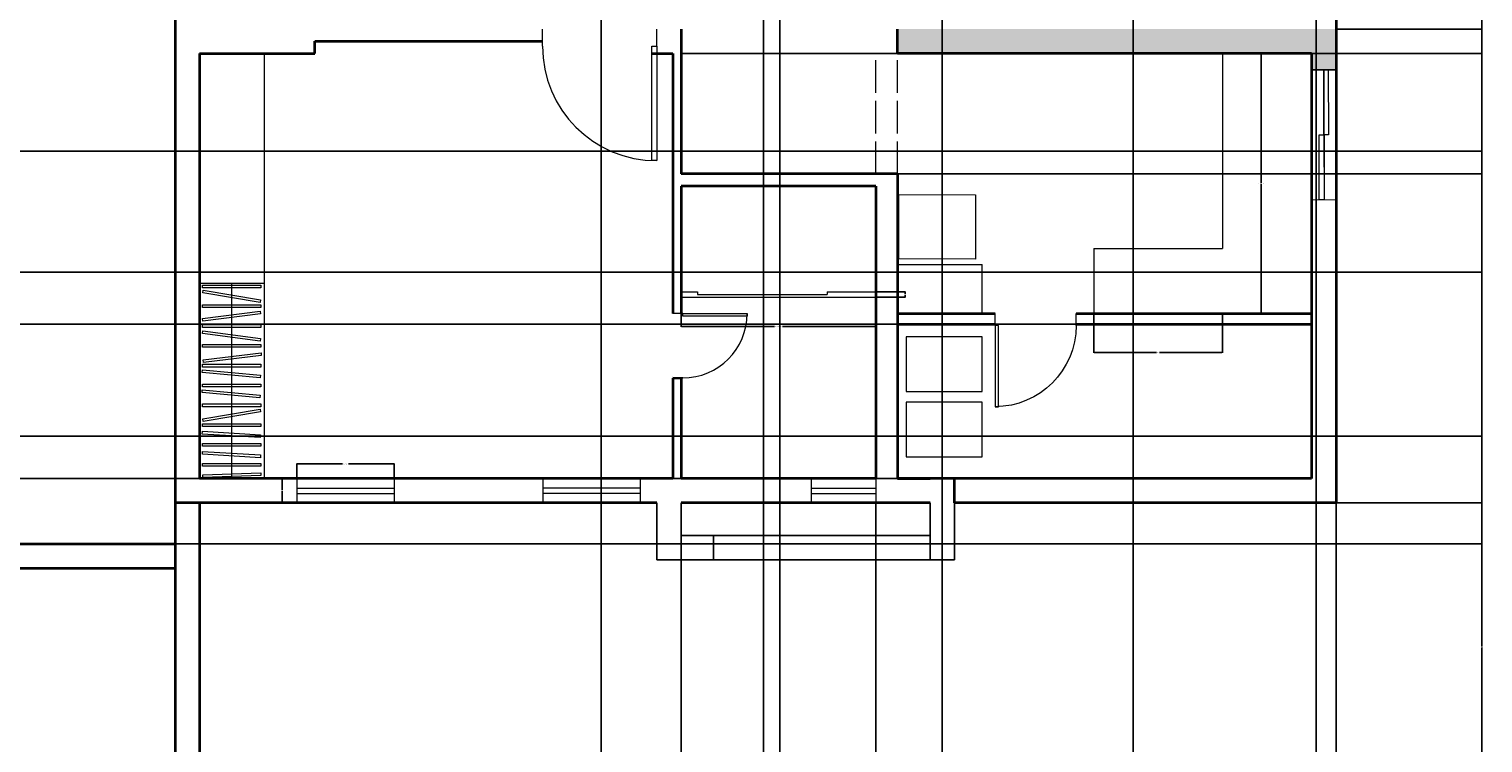
# Model space of a CAD drawing. Units: inches. Extents: x 531915 to 533151, y 849859 to 851471.
# Tile 6 of 7: x 532614 to 533151, y 850858 to 851121. Entities that reach past the tile are written whole.
import ezdxf

# ---------------------------------------------------------------- set-up
doc = ezdxf.new("R2010")
doc.units = ezdxf.units.IN
doc.linetypes.add('ACAD_ISO02W100', pattern=[15, 12, -3])
for name, color, linetype, lineweight in [('A-ANNO-DIMS', 2, 'Continuous', 18), ('A-DOOR', 3, 'Continuous', 18), ('A-FLOR-CASE', 9, 'Continuous', 18), ('A-FLOR-FIXT', 8, 'Continuous', 18), ('A-FLOR-SLAB', 7, 'Continuous', 25), ('A-FURN', 8, 'Continuous', 13), ('A-GLAZ', 4, 'Continuous', 18), ('A-WALL', 7, 'Continuous', 35), ('A-WALL-OVHD', 7, 'ACAD_ISO02W100', 18), ('A-WALL-PATT', 8, 'Continuous', 13)]:
    doc.layers.add(name, color=color, linetype=linetype, lineweight=lineweight)
doc.styles.get("Standard").update_dxf_attribs({"font": 'arial.ttf'})
doc.dimstyles.get("Standard").update_dxf_attribs({"dimtxt": 0.18, "dimasz": 0.18, "dimexe": 0.18, "dimexo": 0.0625, "dimgap": 0.09, "dimtad": 0, "dimtih": 1, "dimtoh": 1, "dimdec": 4, "dimzin": 0, "dimdsep": 46, "dimtxsty": 'Standard', "dimcen": 0.09, "dimadec": 0, "dimazin": 0, "dimtfac": 1, "dimtdec": 4, "dimtofl": 0, "dimtmove": 0, "dimatfit": 3, "dimfxl": 1, "dimtolj": 1, "dimtzin": 0, "dimarcsym": 0})

# ---------------------------------------------------------------- blocks, each defined once
blk = doc.blocks.new('*U2')
for p, q in [((0, 0), (0, -6)), ((40, 0), (40, -6))]:
    blk.add_line(p, q)
blk.add_lwpolyline([(0, 0), (0, 40), (1.75, 40), (1.75, 0)], close=True)
blk.add_arc((0, 0), 40, 0, 90)
blk = doc.blocks.new('WARDROBE-72')
blk.add_line((12, 0), (12, 72))
for points in [[(24, 0), (24, 72), (0, 72), (0, 0)], [(1.15, 70.47), (1.15, 71.48), (22.64, 71.48), (22.64, 70.47)], [(1.21, 68.56), (1.37, 69.55), (22.58, 66.07), (22.41, 65.07)], [(1.15, 63.15), (1.15, 64.16), (22.64, 64.16), (22.64, 63.15)], [(1.3, 58.13), (1.17, 59.13), (22.48, 61.86), (22.61, 60.86)], [(1.11, 53.59), (1.24, 54.59), (22.54, 51.79), (22.41, 50.79)], [(1.15, 55.83), (1.15, 56.84), (22.64, 56.84), (22.64, 55.83)], [(1.15, 48.51), (1.15, 49.52), (22.64, 49.52), (22.64, 48.51)], [(1.55, 42.84), (1.42, 43.84), (22.76, 46.42), (22.88, 45.42)], [(1.04, 39.13), (1.13, 40.14), (22.52, 38.16), (22.43, 37.15)], [(1.15, 41.19), (1.15, 42.2), (22.64, 42.2), (22.64, 41.19)], [(0.98, 31.76), (1.07, 32.76), (22.47, 30.78), (22.37, 29.78)], [(1.15, 33.87), (1.15, 34.88), (22.64, 34.88), (22.64, 33.87)], [(1.15, 26.55), (1.15, 27.56), (22.64, 27.56), (22.64, 26.55)], [(1.38, 21.1), (1.21, 22.1), (22.4, 25.68), (22.57, 24.68)], [(1.05, 16.46), (1.11, 17.47), (22.56, 16.21), (22.5, 15.2)], [(1.15, 19.23), (1.15, 20.24), (22.64, 20.24), (22.64, 19.23)], [(1.15, 11.91), (1.15, 12.92), (22.64, 12.92), (22.64, 11.91)], [(1.11, 8.97), (1.17, 9.98), (22.62, 8.71), (22.56, 7.7)], [(1.15, 4.59), (1.15, 5.6), (22.64, 5.6), (22.64, 4.59)], [(1.25, 0.42), (1.22, 1.43), (22.7, 2.11), (22.73, 1.1)]]:
    blk.add_lwpolyline(points, close=True)
blk = doc.blocks.new('WINDOW-SLIDING-48')
for p, q in [((0, 9), (0, 0)), ((48, 9), (48, 0)), ((0, 4.5), (48, 4.5))]:
    blk.add_line(p, q)
for points in [[(24, 4.5), (48, 4.5), (48, 6.29), (24, 6.29)], [(24, 4.5), (0, 4.5), (0, 2.84), (24, 2.84)]]:
    blk.add_lwpolyline(points, close=True)
blk = doc.blocks.new('UTILITY-FIXTURES-PAIR')
for points in [[(0, 24.11), (28.12, 24.11), (28.12, 44.31), (0, 44.31)], [(0, 0), (28.12, 0), (28.12, 20.2), (0, 20.2)]]:
    blk.add_lwpolyline(points, close=True)
blk = doc.blocks.new('SLIDING-PANEL-72')
for p, q in [((0, 2), (6, 2)), ((6, 2), (6, 1)), ((6, 1), (54, 1)), ((54, 2), (72, 2)), ((54, 2), (54, 1)), ((0, 0), (72, 0))]:
    blk.add_line(p, q)
blk = doc.blocks.new('WINDOW-36')
for p, q in [((0, 9), (0, 0)), ((0, 5.5), (36, 5.5)), ((36, 9), (36, 0)), ((0, 3.5), (36, 3.5))]:
    blk.add_line(p, q)
blk = doc.blocks.new('COUNTER-L-RETURN')
for p, q in [((47.51, 96), (47.51, 24)), ((0, 24), (47.51, 24)), ((0, 24), (0, 0))]:
    blk.add_line(p, q)
blk = doc.blocks.new('COUNTER-END-RETURN')
for p in [(0, 18), (31.29, 0)]:
    blk.add_line(p, (31.29, 18))
blk = doc.blocks.new('*D25')
at = {"layer": 'A-ANNO-DIMS', "color": 0, "lineweight": -2, "transparency": 16777216}
for p, q in [((533054.87, 851112.37), (533069.38, 851112.37)), ((533069.2, 851112.19), (533069.2, 851064.56)), ((533069.2, 851016.55), (533069.2, 851064.19)), ((533054.87, 851016.37), (533069.38, 851016.37))]:
    blk.add_line(p, q, dxfattribs=at)
at = {"layer": 'A-ANNO-DIMS', "color": 0, "transparency": 16777216}
for points in [[(533069.17, 851112.19), (533069.23, 851112.19), (533069.2, 851112.37)], [(533069.17, 851016.55), (533069.23, 851016.55), (533069.2, 851016.37)]]:
    blk.add_solid(points, dxfattribs=at)
at = {"layer": 'Defpoints', "color": 0, "transparency": 16777216}
for p in [(533054.8, 851112.37), (533069.2, 851112.37), (533054.8, 851016.37)]:
    blk.add_point(p, dxfattribs=at)
at = {"layer": 'A-ANNO-DIMS', "color": 0, "transparency": 16777216, "insert": (533069.2, 851064.37), "char_height": 0.18, "attachment_point": 5}
blk.add_mtext('\\A1;L-COUNTER 96 TYP.', dxfattribs=at)
blk = doc.blocks.new('*D26')
at = {"layer": 'A-ANNO-DIMS', "color": 0, "lineweight": -2, "transparency": 16777216}
for p, q in [((533007.29, 851016.31), (533007.29, 851001.79)), ((533054.8, 851016.31), (533054.8, 851001.79)), ((533007.47, 851001.97), (533030.52, 851001.97)), ((533054.62, 851001.97), (533031.58, 851001.97))]:
    blk.add_line(p, q, dxfattribs=at)
at = {"layer": 'A-ANNO-DIMS', "color": 0, "transparency": 16777216}
for points in [[(533007.47, 851002), (533007.47, 851001.94), (533007.29, 851001.97)], [(533054.62, 851002), (533054.62, 851001.94), (533054.8, 851001.97)]]:
    blk.add_solid(points, dxfattribs=at)
at = {"layer": 'Defpoints', "color": 0, "transparency": 16777216}
for p in [(533007.29, 851016.37), (533054.8, 851016.37), (533054.8, 851001.97)]:
    blk.add_point(p, dxfattribs=at)
at = {"layer": 'A-ANNO-DIMS', "color": 0, "transparency": 16777216, "insert": (533031.05, 851001.97), "char_height": 0.18, "attachment_point": 5}
blk.add_mtext('\\A1;48 TYP.', dxfattribs=at)
blk = doc.blocks.new('*D31')
at = {"layer": 'A-ANNO-DIMS', "color": 0, "lineweight": -2, "transparency": 16777216}
for p, q in [((532854.8, 851022.31), (532854.8, 851011.39)), ((532926.8, 851022.31), (532926.8, 851011.39)), ((532854.98, 851011.57), (532889.29, 851011.57)), ((532926.62, 851011.57), (532892.32, 851011.57))]:
    blk.add_line(p, q, dxfattribs=at)
at = {"layer": 'A-ANNO-DIMS', "color": 0, "transparency": 16777216}
for points in [[(532854.98, 851011.6), (532854.98, 851011.54), (532854.8, 851011.57)], [(532926.62, 851011.6), (532926.62, 851011.54), (532926.8, 851011.57)]]:
    blk.add_solid(points, dxfattribs=at)
at = {"layer": 'Defpoints', "color": 0, "transparency": 16777216}
for p in [(532854.8, 851022.37), (532926.8, 851022.37), (532926.8, 851011.57)]:
    blk.add_point(p, dxfattribs=at)
at = {"layer": 'A-ANNO-DIMS', "color": 0, "transparency": 16777216, "insert": (532890.8, 851011.57), "char_height": 0.18, "attachment_point": 5}
blk.add_mtext('\\A1;SLIDING PANEL 72 TYP.', dxfattribs=at)
blk = doc.blocks.new('*D32')
at = {"layer": 'A-ANNO-DIMS', "color": 0, "lineweight": -2, "transparency": 16777216}
for p, q in [((532926.87, 851024.37), (532937.78, 851024.37)), ((532926.87, 851022.37), (532937.78, 851022.37)), ((532937.6, 851024.19), (532937.6, 851023.55)), ((532937.6, 851022.55), (532937.6, 851023.19))]:
    blk.add_line(p, q, dxfattribs=at)
at = {"layer": 'A-ANNO-DIMS', "color": 0, "transparency": 16777216}
for points in [[(532937.57, 851024.19), (532937.63, 851024.19), (532937.6, 851024.37)], [(532937.57, 851022.55), (532937.63, 851022.55), (532937.6, 851022.37)]]:
    blk.add_solid(points, dxfattribs=at)
at = {"layer": 'Defpoints', "color": 0, "transparency": 16777216}
for p in [(532926.8, 851024.37), (532926.8, 851022.37), (532937.6, 851024.37)]:
    blk.add_point(p, dxfattribs=at)
at = {"layer": 'A-ANNO-DIMS', "color": 0, "transparency": 16777216, "insert": (532937.6, 851023.37), "char_height": 0.18, "attachment_point": 5}
blk.add_mtext('\\A1;2 TYP.', dxfattribs=at)
blk = doc.blocks.new('*D33')
at = {"layer": 'A-ANNO-DIMS', "color": 0, "lineweight": -2, "transparency": 16777216}
for p, q in [((532712.8, 850955.44), (532712.8, 850960.95)), ((532712.98, 850960.77), (532729.69, 850960.77)), ((532748.62, 850960.77), (532731.92, 850960.77)), ((532748.8, 850955.44), (532748.8, 850960.95))]:
    blk.add_line(p, q, dxfattribs=at)
at = {"layer": 'A-ANNO-DIMS', "color": 0, "transparency": 16777216}
for points in [[(532712.98, 850960.8), (532712.98, 850960.74), (532712.8, 850960.77)], [(532748.62, 850960.8), (532748.62, 850960.74), (532748.8, 850960.77)]]:
    blk.add_solid(points, dxfattribs=at)
at = {"layer": 'Defpoints', "color": 0, "transparency": 16777216}
for p in [(532748.8, 850960.77), (532712.8, 850955.37), (532748.8, 850955.37)]:
    blk.add_point(p, dxfattribs=at)
at = {"layer": 'A-ANNO-DIMS', "color": 0, "transparency": 16777216, "insert": (532730.8, 850960.77), "char_height": 0.18, "attachment_point": 5}
blk.add_mtext('\\A1;WINDOW 36 TYP.', dxfattribs=at)
blk = doc.blocks.new('*D34')
at = {"layer": 'A-ANNO-DIMS', "color": 0, "lineweight": -2, "transparency": 16777216}
for p, q in [((532712.74, 850955.37), (532707.22, 850955.37)), ((532707.4, 850955.19), (532707.4, 850951.06)), ((532707.4, 850946.55), (532707.4, 850950.69)), ((532712.74, 850946.37), (532707.22, 850946.37))]:
    blk.add_line(p, q, dxfattribs=at)
at = {"layer": 'A-ANNO-DIMS', "color": 0, "transparency": 16777216}
for points in [[(532707.37, 850955.19), (532707.43, 850955.19), (532707.4, 850955.37)], [(532707.37, 850946.55), (532707.43, 850946.55), (532707.4, 850946.37)]]:
    blk.add_solid(points, dxfattribs=at)
at = {"layer": 'Defpoints', "color": 0, "transparency": 16777216}
for p in [(532707.4, 850955.37), (532712.8, 850955.37), (532712.8, 850946.37)]:
    blk.add_point(p, dxfattribs=at)
at = {"layer": 'A-ANNO-DIMS', "color": 0, "transparency": 16777216, "insert": (532707.4, 850950.87), "char_height": 0.18, "attachment_point": 5}
blk.add_mtext('\\A1;9 TYP.', dxfattribs=at)
blk = doc.blocks.new('*D38')
at = {"layer": 'A-ANNO-DIMS', "color": 0, "lineweight": -2, "transparency": 16777216}
for p, q in [((533096.87, 851416.87), (533150.9, 851416.87)), ((533150.72, 851416.69), (533150.72, 850893.31)), ((533150.72, 850369.55), (533150.72, 850892.94)), ((533056.87, 850369.37), (533150.9, 850369.37))]:
    blk.add_line(p, q, dxfattribs=at)
at = {"layer": 'A-ANNO-DIMS', "color": 0, "transparency": 16777216}
for points in [[(533150.69, 851416.69), (533150.75, 851416.69), (533150.72, 851416.87)], [(533150.69, 850369.55), (533150.75, 850369.55), (533150.72, 850369.37)]]:
    blk.add_solid(points, dxfattribs=at)
at = {"layer": 'Defpoints', "color": 0, "transparency": 16777216}
for p in [(533096.8, 851416.87), (533056.8, 850369.37), (533150.72, 850369.37)]:
    blk.add_point(p, dxfattribs=at)
at = {"layer": 'A-ANNO-DIMS', "color": 0, "transparency": 16777216, "insert": (533150.72, 850893.12), "char_height": 0.18, "attachment_point": 5}
blk.add_mtext('\\A1;1047.5', dxfattribs=at)
blk = doc.blocks.new('*D47')
at = {"layer": 'A-ANNO-DIMS', "color": 0, "lineweight": -2, "transparency": 16777216}
for p, q in [((533096.8, 850946.31), (533096.8, 850315.34)), ((533056.8, 850826.31), (533056.8, 850315.34)), ((533056.98, 850315.52), (533076.58, 850315.52)), ((533096.62, 850315.52), (533077.03, 850315.52))]:
    blk.add_line(p, q, dxfattribs=at)
at = {"layer": 'A-ANNO-DIMS', "color": 0, "transparency": 16777216}
for points in [[(533056.98, 850315.55), (533056.98, 850315.49), (533056.8, 850315.52)], [(533096.62, 850315.55), (533096.62, 850315.49), (533096.8, 850315.52)]]:
    blk.add_solid(points, dxfattribs=at)
at = {"layer": 'Defpoints', "color": 0, "transparency": 16777216}
for p in [(533096.8, 850946.37), (533056.8, 850826.37), (533056.8, 850315.52)]:
    blk.add_point(p, dxfattribs=at)
at = {"layer": 'A-ANNO-DIMS', "color": 0, "transparency": 16777216, "insert": (533076.8, 850315.52), "char_height": 0.18, "attachment_point": 5}
blk.add_mtext('\\A1;40', dxfattribs=at)
blk = doc.blocks.new('*D49')
at = {"layer": 'A-ANNO-DIMS', "color": 0, "lineweight": -2, "transparency": 16777216}
for p, q in [((532825.3, 851312.76), (532825.3, 850315.34)), ((532885.3, 851312.76), (532885.3, 850315.34)), ((532825.48, 850315.52), (532855.09, 850315.52)), ((532885.12, 850315.52), (532855.52, 850315.52))]:
    blk.add_line(p, q, dxfattribs=at)
at = {"layer": 'A-ANNO-DIMS', "color": 0, "transparency": 16777216}
for points in [[(532825.48, 850315.55), (532825.48, 850315.49), (532825.3, 850315.52)], [(532885.12, 850315.55), (532885.12, 850315.49), (532885.3, 850315.52)]]:
    blk.add_solid(points, dxfattribs=at)
at = {"layer": 'Defpoints', "color": 0, "transparency": 16777216}
for p in [(532825.3, 851312.82), (532885.3, 851312.82), (532885.3, 850315.52)]:
    blk.add_point(p, dxfattribs=at)
at = {"layer": 'A-ANNO-DIMS', "color": 0, "transparency": 16777216, "insert": (532855.3, 850315.52), "char_height": 0.18, "attachment_point": 5}
blk.add_mtext('\\A1;60', dxfattribs=at)
blk = doc.blocks.new('*D50')
at = {"layer": 'A-ANNO-DIMS', "color": 0, "lineweight": -2, "transparency": 16777216}
for p, q in [((532891.3, 851312.76), (532891.3, 850315.34)), ((532951.3, 851312.76), (532951.3, 850315.34)), ((532891.48, 850315.52), (532921.09, 850315.52)), ((532951.12, 850315.52), (532921.52, 850315.52))]:
    blk.add_line(p, q, dxfattribs=at)
at = {"layer": 'A-ANNO-DIMS', "color": 0, "transparency": 16777216}
for points in [[(532891.48, 850315.55), (532891.48, 850315.49), (532891.3, 850315.52)], [(532951.12, 850315.55), (532951.12, 850315.49), (532951.3, 850315.52)]]:
    blk.add_solid(points, dxfattribs=at)
at = {"layer": 'Defpoints', "color": 0, "transparency": 16777216}
for p in [(532891.3, 851312.82), (532951.3, 851312.82), (532951.3, 850315.52)]:
    blk.add_point(p, dxfattribs=at)
at = {"layer": 'A-ANNO-DIMS', "color": 0, "transparency": 16777216, "insert": (532921.3, 850315.52), "char_height": 0.18, "attachment_point": 5}
blk.add_mtext('\\A1;60', dxfattribs=at)
blk = doc.blocks.new('*D54')
at = {"layer": 'A-ANNO-DIMS', "color": 0, "lineweight": -2, "transparency": 16777216}
for p, q in [((533096.87, 851121.37), (533150.9, 851121.37)), ((533150.72, 851121.19), (533150.72, 851034.06)), ((533150.72, 850946.55), (533150.72, 851033.69)), ((533096.87, 850946.37), (533150.9, 850946.37))]:
    blk.add_line(p, q, dxfattribs=at)
at = {"layer": 'A-ANNO-DIMS', "color": 0, "transparency": 16777216}
for points in [[(533150.69, 851121.19), (533150.75, 851121.19), (533150.72, 851121.37)], [(533150.69, 850946.55), (533150.75, 850946.55), (533150.72, 850946.37)]]:
    blk.add_solid(points, dxfattribs=at)
at = {"layer": 'Defpoints', "color": 0, "transparency": 16777216}
for p in [(533096.8, 851121.37), (533096.8, 850946.37), (533150.72, 850946.37)]:
    blk.add_point(p, dxfattribs=at)
at = {"layer": 'A-ANNO-DIMS', "color": 0, "transparency": 16777216, "insert": (533150.72, 851033.87), "char_height": 0.18, "attachment_point": 5}
blk.add_mtext('\\A1;175', dxfattribs=at)
blk = doc.blocks.new('*D55')
at = {"layer": 'A-ANNO-DIMS', "color": 0, "lineweight": -2, "transparency": 16777216}
for p, q in [((532667.8, 850946.31), (532667.8, 850315.34)), ((532854.8, 850946.31), (532854.8, 850315.34)), ((532667.98, 850315.52), (532761.02, 850315.52)), ((532854.62, 850315.52), (532761.59, 850315.52))]:
    blk.add_line(p, q, dxfattribs=at)
at = {"layer": 'A-ANNO-DIMS', "color": 0, "transparency": 16777216}
for points in [[(532667.98, 850315.55), (532667.98, 850315.49), (532667.8, 850315.52)], [(532854.62, 850315.55), (532854.62, 850315.49), (532854.8, 850315.52)]]:
    blk.add_solid(points, dxfattribs=at)
at = {"layer": 'Defpoints', "color": 0, "transparency": 16777216}
for p in [(532667.8, 850946.37), (532854.8, 850946.37), (532854.8, 850315.52)]:
    blk.add_point(p, dxfattribs=at)
at = {"layer": 'A-ANNO-DIMS', "color": 0, "transparency": 16777216, "insert": (532761.3, 850315.52), "char_height": 0.18, "attachment_point": 5}
blk.add_mtext('\\A1;187', dxfattribs=at)
blk = doc.blocks.new('*D56')
at = {"layer": 'A-ANNO-DIMS', "color": 0, "lineweight": -2, "transparency": 16777216}
for p, q in [((532854.8, 850946.31), (532854.8, 850315.34)), ((532926.8, 850946.31), (532926.8, 850315.34)), ((532854.98, 850315.52), (532890.59, 850315.52)), ((532926.62, 850315.52), (532891.02, 850315.52))]:
    blk.add_line(p, q, dxfattribs=at)
at = {"layer": 'A-ANNO-DIMS', "color": 0, "transparency": 16777216}
for points in [[(532854.98, 850315.55), (532854.98, 850315.49), (532854.8, 850315.52)], [(532926.62, 850315.55), (532926.62, 850315.49), (532926.8, 850315.52)]]:
    blk.add_solid(points, dxfattribs=at)
at = {"layer": 'Defpoints', "color": 0, "transparency": 16777216}
for p in [(532854.8, 850946.37), (532926.8, 850946.37), (532926.8, 850315.52)]:
    blk.add_point(p, dxfattribs=at)
at = {"layer": 'A-ANNO-DIMS', "color": 0, "transparency": 16777216, "insert": (532890.8, 850315.52), "char_height": 0.18, "attachment_point": 5}
blk.add_mtext('\\A1;72', dxfattribs=at)
blk = doc.blocks.new('*D57')
at = {"layer": 'A-ANNO-DIMS', "color": 0, "lineweight": -2, "transparency": 16777216}
for p, q in [((532926.8, 850946.31), (532926.8, 850315.34)), ((533096.8, 850946.31), (533096.8, 850315.34)), ((532926.98, 850315.52), (533011.52, 850315.52)), ((533096.62, 850315.52), (533012.08, 850315.52))]:
    blk.add_line(p, q, dxfattribs=at)
at = {"layer": 'A-ANNO-DIMS', "color": 0, "transparency": 16777216}
for points in [[(532926.98, 850315.55), (532926.98, 850315.49), (532926.8, 850315.52)], [(533096.62, 850315.55), (533096.62, 850315.49), (533096.8, 850315.52)]]:
    blk.add_solid(points, dxfattribs=at)
at = {"layer": 'Defpoints', "color": 0, "transparency": 16777216}
for p in [(532926.8, 850946.37), (533096.8, 850946.37), (533096.8, 850315.52)]:
    blk.add_point(p, dxfattribs=at)
at = {"layer": 'A-ANNO-DIMS', "color": 0, "transparency": 16777216, "insert": (533011.8, 850315.52), "char_height": 0.18, "attachment_point": 5}
blk.add_mtext('\\A1;170', dxfattribs=at)
blk = doc.blocks.new('*D58')
at = {"layer": 'A-ANNO-DIMS', "color": 0, "lineweight": -2, "transparency": 16777216}
for p, q in [((533021.8, 851259.31), (533021.8, 850315.34)), ((533089.48, 851257.99), (533089.48, 850315.34)), ((533021.98, 850315.52), (533055.25, 850315.52)), ((533089.3, 850315.52), (533056.04, 850315.52))]:
    blk.add_line(p, q, dxfattribs=at)
at = {"layer": 'A-ANNO-DIMS', "color": 0, "transparency": 16777216}
for points in [[(533021.98, 850315.55), (533021.98, 850315.49), (533021.8, 850315.52)], [(533089.3, 850315.55), (533089.3, 850315.49), (533089.48, 850315.52)]]:
    blk.add_solid(points, dxfattribs=at)
at = {"layer": 'Defpoints', "color": 0, "transparency": 16777216}
for p in [(533021.8, 851259.37), (533089.48, 851258.05), (533089.48, 850315.52)]:
    blk.add_point(p, dxfattribs=at)
at = {"layer": 'A-ANNO-DIMS', "color": 0, "transparency": 16777216, "insert": (533055.64, 850315.52), "char_height": 0.18, "attachment_point": 5}
blk.add_mtext('\\A1;67.67', dxfattribs=at)
blk = doc.blocks.new('*D59')
at = {"layer": 'A-ANNO-DIMS', "color": 0, "lineweight": -2, "transparency": 16777216}
for p, q in [((533087.74, 851012.37), (531968.71, 851012.37)), ((531968.89, 851012.19), (531968.89, 850984.06)), ((531968.89, 850955.55), (531968.89, 850983.69)), ((533087.74, 850955.37), (531968.71, 850955.37))]:
    blk.add_line(p, q, dxfattribs=at)
at = {"layer": 'A-ANNO-DIMS', "color": 0, "transparency": 16777216}
for points in [[(531968.86, 851012.19), (531968.92, 851012.19), (531968.89, 851012.37)], [(531968.86, 850955.55), (531968.92, 850955.55), (531968.89, 850955.37)]]:
    blk.add_solid(points, dxfattribs=at)
at = {"layer": 'Defpoints', "color": 0, "transparency": 16777216}
for p in [(533087.8, 851012.37), (531968.89, 850955.37), (533087.8, 850955.37)]:
    blk.add_point(p, dxfattribs=at)
at = {"layer": 'A-ANNO-DIMS', "color": 0, "transparency": 16777216, "insert": (531968.89, 850983.87), "char_height": 0.18, "attachment_point": 5}
blk.add_mtext('\\A1;57', dxfattribs=at)
blk = doc.blocks.new('*D71')
at = {"layer": 'A-ANNO-DIMS', "color": 0, "lineweight": -2, "transparency": 16777216}
for p, q in [((532589.8, 850931.17), (532589.8, 850315.34)), ((532667.8, 850931.17), (532667.8, 850315.34)), ((532589.98, 850315.52), (532628.59, 850315.52)), ((532667.62, 850315.52), (532629.02, 850315.52))]:
    blk.add_line(p, q, dxfattribs=at)
at = {"layer": 'A-ANNO-DIMS', "color": 0, "transparency": 16777216}
for points in [[(532589.98, 850315.55), (532589.98, 850315.49), (532589.8, 850315.52)], [(532667.62, 850315.55), (532667.62, 850315.49), (532667.8, 850315.52)]]:
    blk.add_solid(points, dxfattribs=at)
at = {"layer": 'Defpoints', "color": 0, "transparency": 16777216}
for p in [(532589.8, 850931.23), (532667.8, 850931.23), (532667.8, 850315.52)]:
    blk.add_point(p, dxfattribs=at)
at = {"layer": 'A-ANNO-DIMS', "color": 0, "transparency": 16777216, "insert": (532628.8, 850315.52), "char_height": 0.18, "attachment_point": 5}
blk.add_mtext('\\A1;78', dxfattribs=at)
blk = doc.blocks.new('*D74')
at = {"layer": 'A-ANNO-DIMS', "color": 0, "lineweight": -2, "transparency": 16777216}
for p, q in [((532580.87, 850971.01), (533150.9, 850971.01)), ((533150.72, 850970.83), (533150.72, 850951.31)), ((533150.72, 850931.41), (533150.72, 850950.94)), ((532580.87, 850931.23), (533150.9, 850931.23))]:
    blk.add_line(p, q, dxfattribs=at)
at = {"layer": 'A-ANNO-DIMS', "color": 0, "transparency": 16777216}
for points in [[(533150.69, 850970.83), (533150.75, 850970.83), (533150.72, 850971.01)], [(533150.69, 850931.41), (533150.75, 850931.41), (533150.72, 850931.23)]]:
    blk.add_solid(points, dxfattribs=at)
at = {"layer": 'Defpoints', "color": 0, "transparency": 16777216}
for p in [(532580.8, 850971.01), (533150.72, 850971.01), (532580.8, 850931.23)]:
    blk.add_point(p, dxfattribs=at)
at = {"layer": 'A-ANNO-DIMS', "color": 0, "transparency": 16777216, "insert": (533150.72, 850951.12), "char_height": 0.18, "attachment_point": 5}
blk.add_mtext('\\A1;39.78', dxfattribs=at)
blk = doc.blocks.new('*D75')
at = {"layer": 'A-ANNO-DIMS', "color": 0, "lineweight": -2, "transparency": 16777216}
for p, q in [((532580.87, 851031.56), (533150.9, 851031.56)), ((533150.72, 851031.38), (533150.72, 851001.47)), ((533150.72, 850971.19), (533150.72, 851001.11)), ((532580.87, 850971.01), (533150.9, 850971.01))]:
    blk.add_line(p, q, dxfattribs=at)
at = {"layer": 'A-ANNO-DIMS', "color": 0, "transparency": 16777216}
for points in [[(533150.69, 851031.38), (533150.75, 851031.38), (533150.72, 851031.56)], [(533150.69, 850971.19), (533150.75, 850971.19), (533150.72, 850971.01)]]:
    blk.add_solid(points, dxfattribs=at)
at = {"layer": 'Defpoints', "color": 0, "transparency": 16777216}
for p in [(532580.8, 851031.56), (533150.72, 851031.56), (532580.8, 850971.01)]:
    blk.add_point(p, dxfattribs=at)
at = {"layer": 'A-ANNO-DIMS', "color": 0, "transparency": 16777216, "insert": (533150.72, 851001.29), "char_height": 0.18, "attachment_point": 5}
blk.add_mtext('\\A1;60.55', dxfattribs=at)
blk = doc.blocks.new('*D80')
at = {"layer": 'A-ANNO-DIMS', "color": 0, "lineweight": -2, "transparency": 16777216}
for p, q in [((532580.87, 851146.23), (533150.9, 851146.23)), ((533150.72, 851146.05), (533150.72, 851111.42)), ((533150.72, 851076.41), (533150.72, 851111.05)), ((532580.87, 851076.23), (533150.9, 851076.23))]:
    blk.add_line(p, q, dxfattribs=at)
at = {"layer": 'A-ANNO-DIMS', "color": 0, "transparency": 16777216}
for points in [[(533150.69, 851146.05), (533150.75, 851146.05), (533150.72, 851146.23)], [(533150.69, 851076.41), (533150.75, 851076.41), (533150.72, 851076.23)]]:
    blk.add_solid(points, dxfattribs=at)
at = {"layer": 'Defpoints', "color": 0, "transparency": 16777216}
for p in [(532580.8, 851146.23), (532580.8, 851076.23), (533150.72, 851076.23)]:
    blk.add_point(p, dxfattribs=at)
at = {"layer": 'A-ANNO-DIMS', "color": 0, "transparency": 16777216, "insert": (533150.72, 851111.23), "char_height": 0.18, "attachment_point": 5}
blk.add_mtext('\\A1;70', dxfattribs=at)
blk = doc.blocks.new('*D82')
at = {"layer": 'A-ANNO-DIMS', "color": 0, "lineweight": -2, "transparency": 16777216}
for p, q in [((532854.87, 851112.37), (533150.9, 851112.37)), ((533150.72, 851112.19), (533150.72, 851090.31)), ((533150.72, 851068.05), (533150.72, 851089.94)), ((532854.87, 851067.87), (533150.9, 851067.87))]:
    blk.add_line(p, q, dxfattribs=at)
at = {"layer": 'A-ANNO-DIMS', "color": 0, "transparency": 16777216}
for points in [[(533150.69, 851112.19), (533150.75, 851112.19), (533150.72, 851112.37)], [(533150.69, 851068.05), (533150.75, 851068.05), (533150.72, 851067.87)]]:
    blk.add_solid(points, dxfattribs=at)
at = {"layer": 'Defpoints', "color": 0, "transparency": 16777216}
for p in [(532854.8, 851112.37), (532854.8, 851067.87), (533150.72, 851067.87)]:
    blk.add_point(p, dxfattribs=at)
at = {"layer": 'A-ANNO-DIMS', "color": 0, "transparency": 16777216, "insert": (533150.72, 851090.12), "char_height": 0.18, "attachment_point": 5}
blk.add_mtext('\\A1;44.5', dxfattribs=at)

msp = doc.modelspace()

# ---------------------------------------------------------------- hatches: boundary and pattern name
at = {"layer": 'A-WALL-PATT'}
h = msp.add_hatch(color=256, dxfattribs=at)
h.dxf.hatch_style = 1
h.paths.add_polyline_path([(533096.8048, 851121.374), (532951.8048, 851121.374), (532934.8048, 851121.374), (532934.8048, 851112.374), (533087.8048, 851112.374), (533087.8048, 851106.374), (533096.8048, 851106.374)])

# ---------------------------------------------------------------- linework, layer by layer
at = {"layer": 'A-FLOR-FIXT'}
msp.add_lwpolyline([(532935.2845, 851060.2797), (532963.6185, 851060.1571), (532963.6185, 851036.3719), (532935.2845, 851036.4945)], close=True, dxfattribs=at)
at = {"layer": 'A-FLOR-SLAB'}
for p, q in [((532845.8048, 850925.374), (532845.8048, 850946.374)), ((532854.8048, 850946.374), (532854.8048, 850934.374)), ((532946.8048, 850946.374), (532946.8048, 850925.374)), ((532955.8048, 850925.374), (532955.8048, 850946.374)), ((532854.8048, 850934.374), (532866.8048, 850934.374)), ((532866.8048, 850934.374), (532866.8048, 850925.374)), ((532866.8048, 850934.374), (532946.8048, 850934.374)), ((532866.8048, 850925.374), (532845.8048, 850925.374)), ((532866.8048, 850925.374), (532946.8048, 850925.374)), ((532946.8048, 850925.374), (532953.1076, 850925.374)), ((532946.8048, 850925.374), (532955.8048, 850925.374))]:
    msp.add_line(p, q, dxfattribs=at)
at = {"layer": 'A-FURN'}
msp.add_line((532700.8048, 851027.374), (532700.8048, 851112.374), dxfattribs=at)
at = {"layer": 'A-GLAZ'}
for p, q in [((533096.8048, 851106.374), (533087.8048, 851106.374)), ((532902.8048, 850955.374), (532902.8048, 850946.374)), ((532902.8048, 850951.874), (532926.8048, 850951.874)), ((532926.8048, 850955.374), (532926.8048, 850946.374)), ((532902.8048, 850949.874), (532926.8048, 850949.874))]:
    msp.add_line(p, q, dxfattribs=at)
at = {"layer": 'A-WALL'}
for p, q in [((533096.8048, 851416.874), (533096.8048, 850946.374)), ((533096.8048, 851416.874), (533096.8048, 850946.374)), ((532667.8048, 851211.374), (532667.8048, 850946.374)), ((532667.8048, 851211.374), (532667.8048, 850369.374)), ((532719.4067, 851112.374), (532719.4067, 851116.874)), ((532719.4067, 851116.874), (532803.553, 851116.874)), ((532854.8048, 851121.374), (532854.8048, 851067.874)), ((532934.8048, 851112.374), (532934.8048, 851121.374)), ((532676.8048, 851112.374), (532719.4067, 851112.374)), ((532676.8048, 851112.374), (532676.8048, 850955.374)), ((532676.8048, 851112.374), (532676.8048, 850955.374)), ((532843.9563, 851112.374), (532851.8048, 851112.374)), ((532851.8048, 851112.374), (532851.8048, 851016.374)), ((533087.8048, 851112.374), (532934.8048, 851112.374)), ((533087.8048, 851112.374), (533087.8048, 850955.374)), ((532934.8048, 851067.874), (532854.8048, 851067.874)), ((532926.8048, 851063.374), (532854.8048, 851063.374)), ((532854.8048, 851063.374), (532854.8048, 851016.374)), ((532926.8048, 851063.374), (532926.8048, 850955.374)), ((532934.8048, 851067.874), (532934.8048, 850955.374)), ((532934.8048, 851016.374), (532970.8048, 851016.374)), ((533000.7592, 851016.374), (533087.8048, 851016.374)), ((532934.8048, 851012.374), (532970.8048, 851012.374)), ((533000.7592, 851012.374), (533087.8048, 851012.374)), ((532851.8048, 850992.4281), (532851.8048, 850955.374)), ((532854.8048, 850992.374), (532851.8048, 850992.4281)), ((532854.8048, 850992.374), (532854.8048, 850955.374)), ((532851.8048, 850955.374), (532676.8048, 850955.374)), ((532926.8048, 850955.374), (532854.8048, 850955.374)), ((533087.8048, 850955.374), (532934.8048, 850955.374)), ((532934.8048, 850955.374), (532946.8048, 850955.374)), ((532955.8048, 850946.374), (532955.8048, 850955.374)), ((532845.8048, 850946.374), (532667.8048, 850946.374)), ((532676.8048, 850946.374), (532676.8048, 850369.374)), ((532946.8048, 850946.374), (532854.8048, 850946.374)), ((533096.8048, 850946.374), (532955.8048, 850946.374)), ((532451.8048, 850931.2344), (532667.8048, 850931.2344)), ((532667.8048, 850931.2344), (532667.8048, 850369.374)), ((532676.8048, 850931.2344), (532676.8048, 850369.374)), ((532451.8048, 850922.2344), (532667.8048, 850922.2344))]:
    msp.add_line(p, q, dxfattribs=at)
at = {"layer": 'A-WALL-OVHD'}
for p, q in [((532926.8048, 851112.374), (532854.8048, 851112.374)), ((532926.8048, 851067.874), (532926.8048, 851112.374)), ((532934.8048, 851067.874), (532934.8048, 851112.374))]:
    msp.add_line(p, q, dxfattribs=at)

# ---------------------------------------------------------------- block references
at = {"layer": 'A-DOOR'}
for p, xscale, yscale, zscale, rotation in [((532845.8048, 851115.0362), 1.056294156906435, 1.056294156906435, 1.056294156906435, 180), ((532855.3812, 851016.374), 0.596075753296685, 0.596075753296685, 0.596075753296685, 270), ((532970.8048, 851011.8808), -0.7488601199280389, 0.7488601199280389, 0.7488601199280389, 180)]:
    msp.add_blockref('*U2', p, dxfattribs=dict(at, xscale=xscale, yscale=yscale, zscale=zscale, rotation=rotation))
at = {"layer": 'A-FLOR-CASE'}
for name, p in [('COUNTER-L-RETURN', (533007.2933, 851016.374)), ('COUNTER-END-RETURN', (532934.8048, 851016.374))]:
    msp.add_blockref(name, p, dxfattribs=at)
at = {"layer": 'A-FLOR-FIXT'}
msp.add_blockref('UTILITY-FIXTURES-PAIR', (532937.9813, 850963.385), dxfattribs=at)
at = {"layer": 'A-FURN'}
msp.add_blockref('WARDROBE-72', (532676.8048, 850955.374), dxfattribs=at)
at = {"layer": 'A-GLAZ', "extrusion": (0, 0, -1), "zscale": -1, "rotation": 269.9286429430327}
msp.add_blockref('WINDOW-SLIDING-48', (-533096.8058, 851106.3796), dxfattribs=at)
at = {"layer": 'A-GLAZ'}
for name, p in [('SLIDING-PANEL-72', (532854.8048, 851022.374)), ('WINDOW-36', (532712.8048, 850946.374))]:
    msp.add_blockref(name, p, dxfattribs=at)
at = {"layer": 'A-GLAZ', "rotation": 180}
msp.add_blockref('WINDOW-36', (532839.8048, 850955.374), dxfattribs=at)

# ---------------------------------------------------------------- dimensions: what is measured, and where the dimension line sits
at = {"layer": 'A-ANNO-DIMS'}
for base, p1, p2, override, picture, middle in [((533150.7156, 850369.374), (533096.8048, 851416.874), (533056.8048, 850369.374), {"dimdec": 1, "dimlfac": 1, "dimrnd": 0, "dimzin": 0, "dimdsep": 46, "dimlunit": 2}, '*D38', (533150.7156, 850893.124)), ((533150.7156, 851076.2344), (532580.8048, 851146.2344), (532580.8048, 851076.2344), {"dimdec": 0, "dimlfac": 1, "dimrnd": 0, "dimzin": 0, "dimdsep": 46, "dimlunit": 2}, '*D80', (533150.7156, 851111.2344)), ((533150.7156, 850946.374), (533096.8048, 851121.374), (533096.8048, 850946.374), {"dimdec": 0, "dimlfac": 1, "dimrnd": 0, "dimzin": 0, "dimdsep": 46, "dimlunit": 2}, '*D54', (533150.7156, 851033.874)), ((533150.7156, 851067.874), (532854.8048, 851112.374), (532854.8048, 851067.874), {"dimdec": 1, "dimlfac": 1, "dimrnd": 0, "dimzin": 0, "dimdsep": 46, "dimlunit": 2}, '*D82', (533150.7156, 851090.124)), ((533150.7156, 851031.5642), (532580.8048, 850971.0147), (532580.8048, 851031.5642), {"dimdec": 2, "dimlfac": 1, "dimrnd": 0, "dimzin": 0, "dimdsep": 46, "dimlunit": 2}, '*D75', (533150.7156, 851001.2895)), ((531968.8939, 850955.374), (533087.8048, 851012.374), (533087.8048, 850955.374), {"dimdec": 0, "dimlfac": 1, "dimrnd": 0, "dimzin": 0, "dimdsep": 46, "dimlunit": 2}, '*D59', (531968.8939, 850983.874)), ((533150.7156, 850971.0147), (532580.8048, 850931.2344), (532580.8048, 850971.0147), {"dimdec": 2, "dimlfac": 1, "dimrnd": 0, "dimzin": 0, "dimdsep": 46, "dimlunit": 2}, '*D74', (533150.7156, 850951.1246))]:
    dim = msp.add_linear_dim(base=base, p1=p1, p2=p2, angle=90, dimstyle='Standard', override=override, dxfattribs=at)
    dim.commit()
    dim.dimension.update_dxf_attribs({"geometry": picture, "text_midpoint": middle})
for base, p1, p2, override, picture, middle in [((532885.3048, 850315.524), (532825.3048, 851312.8243), (532885.3048, 851312.8243), {"dimdec": 0, "dimlfac": 1, "dimrnd": 0, "dimzin": 0, "dimdsep": 46, "dimlunit": 2}, '*D49', (532855.3048, 850315.524)), ((532951.3048, 850315.524), (532891.3048, 851312.8243), (532951.3048, 851312.8243), {"dimdec": 0, "dimlfac": 1, "dimrnd": 0, "dimzin": 0, "dimdsep": 46, "dimlunit": 2}, '*D50', (532921.3048, 850315.524)), ((533089.477, 850315.524), (533021.8048, 851259.374), (533089.477, 851258.0527), {"dimdec": 2, "dimlfac": 1, "dimrnd": 0, "dimzin": 0, "dimdsep": 46, "dimlunit": 2}, '*D58', (533055.6409, 850315.524)), ((532854.8048, 850315.524), (532667.8048, 850946.374), (532854.8048, 850946.374), {"dimdec": 0, "dimlfac": 1, "dimrnd": 0, "dimzin": 0, "dimdsep": 46, "dimlunit": 2}, '*D55', (532761.3048, 850315.524)), ((532926.8048, 850315.524), (532854.8048, 850946.374), (532926.8048, 850946.374), {"dimdec": 0, "dimlfac": 1, "dimrnd": 0, "dimzin": 0, "dimdsep": 46, "dimlunit": 2}, '*D56', (532890.8048, 850315.524)), ((533096.8048, 850315.524), (532926.8048, 850946.374), (533096.8048, 850946.374), {"dimdec": 0, "dimlfac": 1, "dimrnd": 0, "dimzin": 0, "dimdsep": 46, "dimlunit": 2}, '*D57', (533011.8048, 850315.524)), ((533056.8048, 850315.524), (533096.8048, 850946.374), (533056.8048, 850826.374), {"dimdec": 0, "dimlfac": 1, "dimrnd": 0, "dimzin": 0, "dimdsep": 46, "dimlunit": 2}, '*D47', (533076.8048, 850315.524)), ((532667.8048, 850315.524), (532589.8048, 850931.2344), (532667.8048, 850931.2344), {"dimdec": 0, "dimlfac": 1, "dimrnd": 0, "dimzin": 0, "dimdsep": 46, "dimlunit": 2}, '*D71', (532628.8048, 850315.524))]:
    dim = msp.add_linear_dim(base=base, p1=p1, p2=p2, dimstyle='Standard', override=override, dxfattribs=at)
    dim.commit()
    dim.dimension.update_dxf_attribs({"geometry": picture, "text_midpoint": middle})
for base, p1, p2, text, picture, middle in [((533069.2048, 851112.374), (533054.8048, 851016.374), (533054.8048, 851112.374), 'L-COUNTER <> TYP.', '*D25', (533069.2048, 851064.374)), ((532937.6048, 851024.374), (532926.8048, 851022.374), (532926.8048, 851024.374), '<> TYP.', '*D32', (532937.6048, 851023.374)), ((532707.4048, 850955.374), (532712.8048, 850946.374), (532712.8048, 850955.374), '<> TYP.', '*D34', (532707.4048, 850950.874))]:
    dim = msp.add_linear_dim(base=base, p1=p1, p2=p2, angle=90, text=text, dimstyle='Standard', override={"dimdec": 0, "dimlfac": 1, "dimrnd": 0, "dimzin": 0, "dimdsep": 46, "dimlunit": 2}, dxfattribs=at)
    dim.commit()
    dim.dimension.update_dxf_attribs({"geometry": picture, "text_midpoint": middle})
for base, p1, p2, text, picture, middle in [((532926.8048, 851011.574), (532854.8048, 851022.374), (532926.8048, 851022.374), 'SLIDING PANEL <> TYP.', '*D31', (532890.8048, 851011.574)), ((533054.8048, 851001.974), (533007.2933, 851016.374), (533054.8048, 851016.374), '<> TYP.', '*D26', (533031.049, 851001.974)), ((532748.8048, 850960.774), (532712.8048, 850955.374), (532748.8048, 850955.374), 'WINDOW <> TYP.', '*D33', (532730.8048, 850960.774))]:
    dim = msp.add_linear_dim(base=base, p1=p1, p2=p2, text=text, dimstyle='Standard', override={"dimdec": 0, "dimlfac": 1, "dimrnd": 0, "dimzin": 0, "dimdsep": 46, "dimlunit": 2}, dxfattribs=at)
    dim.commit()
    dim.dimension.update_dxf_attribs({"geometry": picture, "text_midpoint": middle})

doc.saveas('drawing.dxf')
